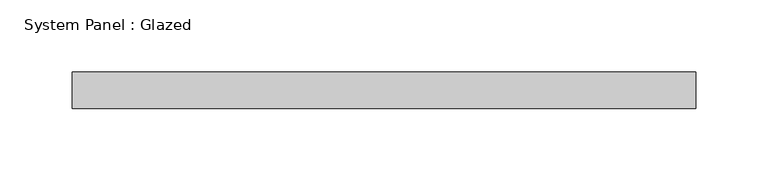
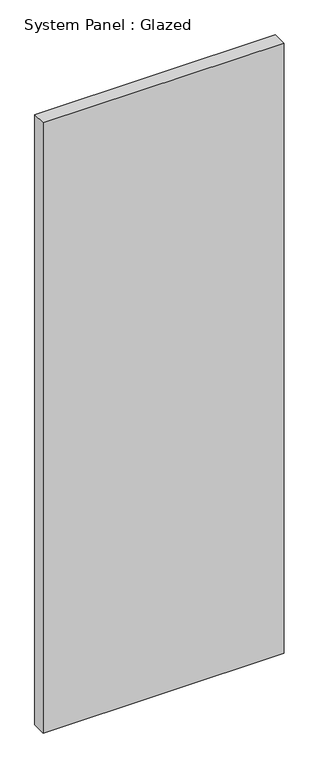
"""IFC4 building model written with IfcOpenShell, lengths in millimetres: plate geometry, System Panel : Glazed."""

from ifc_helpers import new_model, si_unit, origin, origin_with_axes, place, context, project, spatial, polyline, outline, extrude, source, transform, mapped, element, save


def system_panel_glazed_f69cdbc3(model_context):
    return source(origin(), model_context, "Body", "SweptSolid", [
        extrude(outline(polyline([(215.9, 19.05), (-215.9, 19.05), (-215.9, 44.45), (215.9, 44.45), (215.9, 19.05)])), origin_with_axes(), (0.0, 0.0, 1.0), 1155.7),
    ])


if __name__ == "__main__":
    model = new_model("IFC4")
    model_context = context("Model", 3, world=origin())
    ifc_project = project(units=[si_unit("LENGTHUNIT", "METRE", prefix="MILLI")], contexts=[model_context])
    site = spatial("IfcSite", under=ifc_project)
    building = spatial("IfcBuilding", under=site)
    placement = place(None, origin())
    system_panel_glazed_shape = system_panel_glazed_f69cdbc3(model_context)
    element("IfcPlate", 1, ObjectType="System Panel : Glazed", at=placement, inside=building, context=model_context, shape_type="MappedRepresentation", body=[
        mapped(system_panel_glazed_shape, transform((0.0, 0.0, 0.0), x_axis=(1.0, 0.0, 0.0), y_axis=(0.0, 1.0, 0.0), z_axis=(0.0, 0.0, 1.0))),
    ])
    save(model, "model.ifc")

# Revit data of these elements
# Type "System Panel : Glazed"
#   Construction Type Id = "GSP4R"
#   Analytic Construction = "1/8 in Pilkington single glazing"
#   Visual Light Transmittance = 0.9
#   Solar Heat Gain Coefficient = 0.86
#   Heat Transfer Coefficient (U) = 1.18115 BTU/(h·ft²·°F)
# Element 1 (IfcPlate, "System Panel : Glazed")
#   Materials on its faces: "Glass"
# Materials
#   "Glass": class "Glass", colour RGB 0 128 192, transparency 0.75, Description = "Soda Lime Glass", Cost = 0
